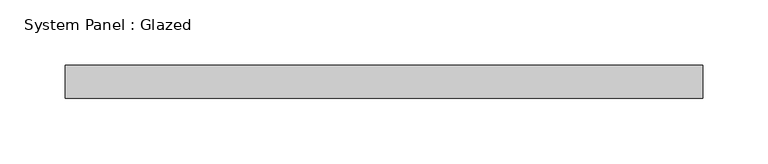
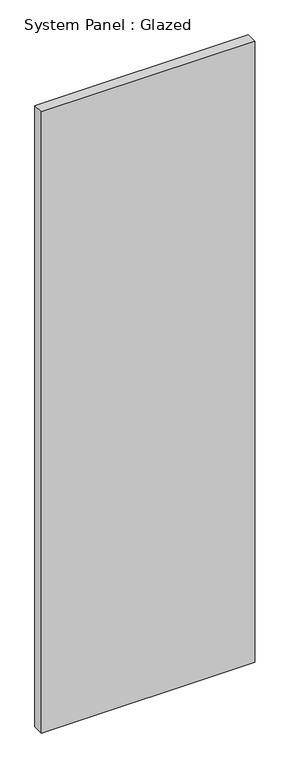
"""IFC4 building model written with IfcOpenShell, lengths in millimetres: plate geometry, System Panel : Glazed."""

from ifc_helpers import new_model, si_unit, origin, origin_with_axes, place, context, project, spatial, polyline, outline, extrude, source, transform, mapped, element, save


def system_panel_glazed_cf012afc(model_context):
    return source(origin(), model_context, "Body", "SweptSolid", [
        extrude(outline(polyline([(244.475, 19.05), (-244.475, 19.05), (-244.475, 44.45), (244.475, 44.45), (244.475, 19.05)])), origin_with_axes(), (0.0, 0.0, 1.0), 1504.45108),
    ])


if __name__ == "__main__":
    model = new_model("IFC4")
    model_context = context("Model", 3, world=origin())
    ifc_project = project(units=[si_unit("LENGTHUNIT", "METRE", prefix="MILLI")], contexts=[model_context])
    site = spatial("IfcSite", under=ifc_project)
    building = spatial("IfcBuilding", under=site)
    placement = place(None, origin())
    system_panel_glazed_shape = system_panel_glazed_cf012afc(model_context)
    element("IfcPlate", 1, ObjectType="System Panel : Glazed", at=placement, inside=building, context=model_context, shape_type="MappedRepresentation", body=[
        mapped(system_panel_glazed_shape, transform((0.0, 0.0, 0.0), x_axis=(1.0, 0.0, 0.0), y_axis=(0.0, 1.0, 0.0), z_axis=(0.0, 0.0, 1.0))),
    ])
    save(model, "model.ifc")

# Revit data of these elements
# Type "System Panel : Glazed"
#   Construction Type Id = "GSP4R"
#   Analytic Construction = "1/8 in Pilkington single glazing"
#   Visual Light Transmittance = 0.9
#   Solar Heat Gain Coefficient = 0.86
#   Heat Transfer Coefficient (U) = 1.18115 BTU/(h·ft²·°F)
#   Define Thermal Properties by = 1
# Element 1 (IfcPlate, "System Panel : Glazed")
#   Materials on its faces: "Glass"
# Materials
#   "Glass": class "Glass", colour RGB 0 128 192, transparency 0.75, Description = "Soda Lime Glass", Cost = 0
